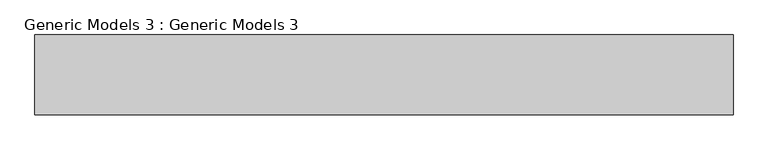
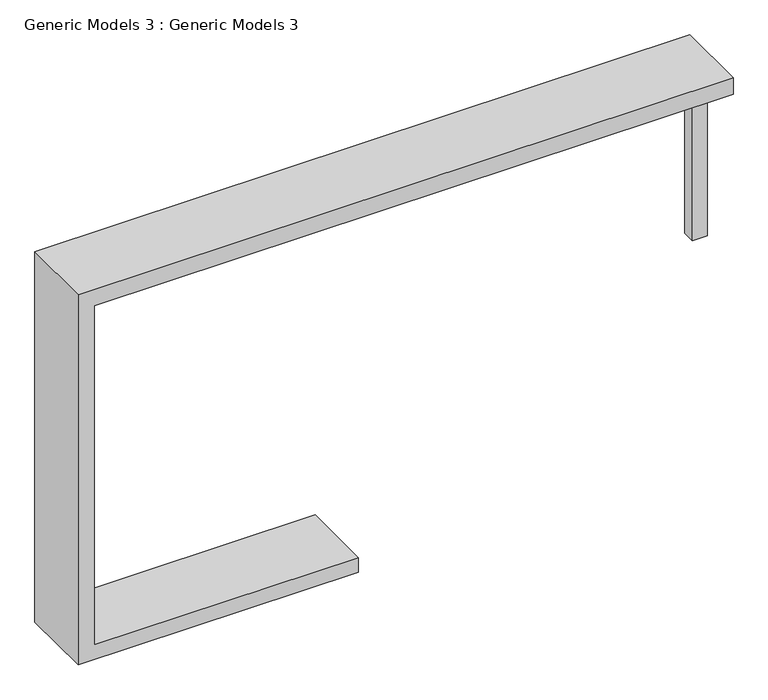
"""IFC4 building model written with IfcOpenShell, lengths in millimetres: proxy geometry, Generic Models 3 : Generic Models 3."""

from ifc_helpers import new_model, si_unit, frame, origin, place, context, project, spatial, polyline, outline, extrude, source, transform, mapped, element, save


def generic_models_3_generic_models_3_3340ffbe(model_context):
    return source(origin(), model_context, "Body", "SweptSolid", [
        extrude(outline(polyline([(-6828.6721594, -15171.132201), (-6828.6721594, -14940.315227), (-6568.540816, -14940.315227), (-6568.540816, -15171.132201), (-6828.6721594, -15171.132201)])), frame((0.0, 0.0, 6429.1436541), z_axis=(0.0, 0.0, 1.0), x_axis=(1.0, 0.0, 0.0)), (0.0, 0.0, 1.0), 2824.9770459),
        extrude(outline(polyline([(9144.0, -6272.2195233), (9448.8, -6272.2195233), (9448.8, -17832.2537599), (2540.9085414, -17832.2537599), (2540.9085414, -12885.8959649), (2812.195855, -12885.8959649), (2812.195855, -17543.4695233), (9144.0, -17543.4695233), (9144.0, -6272.2195233)])), frame((0.0, -15454.2906536, 0.0), z_axis=(0.0, 1.0, 0.0), x_axis=(0.0, 0.0, 1.0)), (0.0, 0.0, 1.0), 1319.5153966),
    ])


if __name__ == "__main__":
    model = new_model("IFC4")
    model_context = context("Model", 3, world=origin())
    ifc_project = project(units=[si_unit("LENGTHUNIT", "METRE", prefix="MILLI")], contexts=[model_context])
    site = spatial("IfcSite", under=ifc_project)
    building = spatial("IfcBuilding", under=site)
    placement = place(None, origin())
    generic_models_3_generic_models_3_shape = generic_models_3_generic_models_3_3340ffbe(model_context)
    element("IfcBuildingElementProxy", 1, Name="Generic Models 3 : Generic Models 3", ObjectType="Generic Models 3 : Generic Models 3", at=placement, inside=building, context=model_context, shape_type="MappedRepresentation", body=[
        mapped(generic_models_3_generic_models_3_shape, transform((0.0, 0.0, 0.0), x_axis=(1.0, 0.0, 0.0), y_axis=(0.0, 1.0, 0.0), z_axis=(0.0, 0.0, 1.0))),
    ])
    save(model, "model.ifc")
